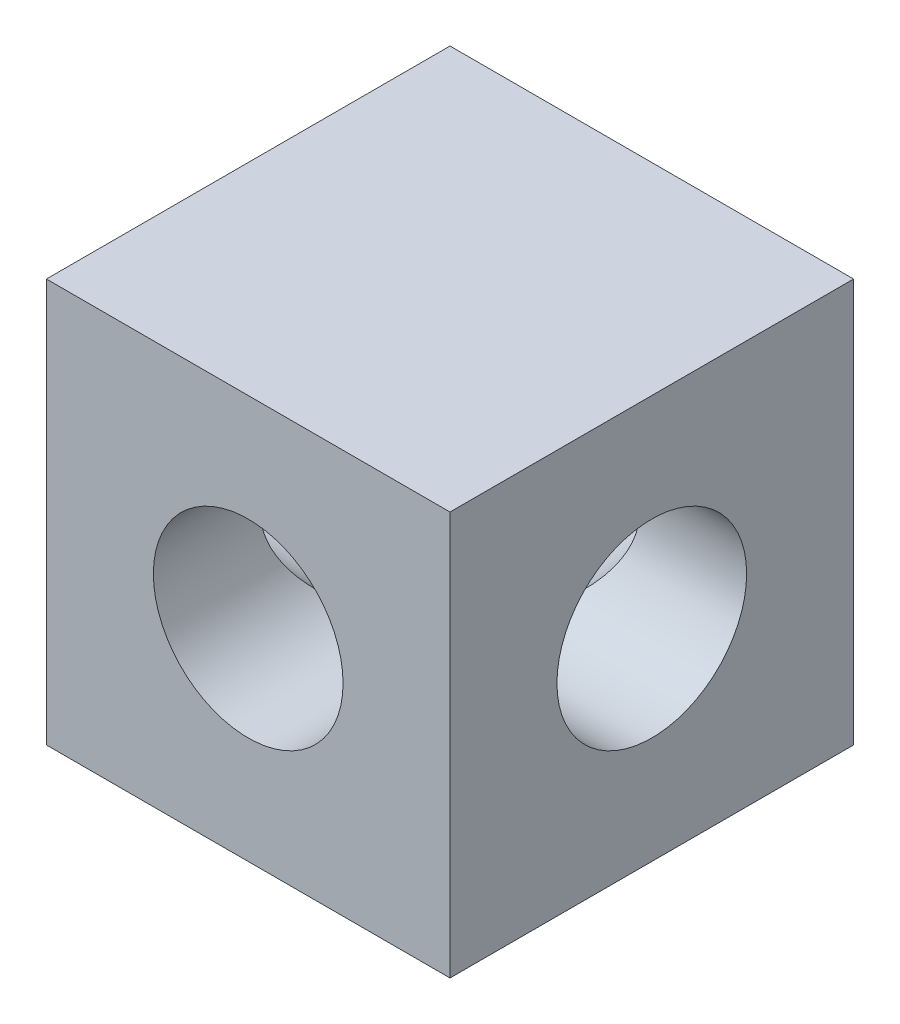
from build123d import *

# Parameters (mm, degrees)
BLOCK_PROFILE_20_32_SQUARE_W = 20.32
BLOCK_PROFILE_20_32_SQUARE_H = 20.32
CUBE_BLOCK_20_32_DEPTH       = 20.32
CROSS_HOLE_A_PROFILE_R       = 4.775
CROSS_HOLE_A_9_35_DEPTH      = 31.48
CROSS_HOLE_B_PROFILE_R       = 4.775
CROSS_HOLE_B_9_35_DEPTH      = 31.48


with BuildPart() as part:
    # Block Profile 20.32 Square → Cube Block 20.32 (new body)
    with BuildSketch(Plane(origin=(0, 0, 0), x_dir=(1, 0, 0), z_dir=(0, 1, 0))):
        Rectangle(BLOCK_PROFILE_20_32_SQUARE_W, BLOCK_PROFILE_20_32_SQUARE_H)
    extrude(amount=CUBE_BLOCK_20_32_DEPTH)

    # Cross Hole A Profile → Cross Hole A Ø9.35 (cut, through all)
    with BuildSketch(Plane.XY.offset(10.16)):
        with Locations((0, 10.16)):
            Circle(CROSS_HOLE_A_PROFILE_R)
    extrude(amount=-CROSS_HOLE_A_9_35_DEPTH, mode=Mode.SUBTRACT)

    # Cross Hole B Profile → Cross Hole B Ø9.35 (cut, through all)
    with BuildSketch(Plane(origin=(10.16, 0, 0), x_dir=(0, 0, -1), z_dir=(1, 0, 0))):
        with Locations((0, 10.16)):
            Circle(CROSS_HOLE_B_PROFILE_R)
    extrude(amount=-CROSS_HOLE_B_9_35_DEPTH, mode=Mode.SUBTRACT)


solid = part.part
